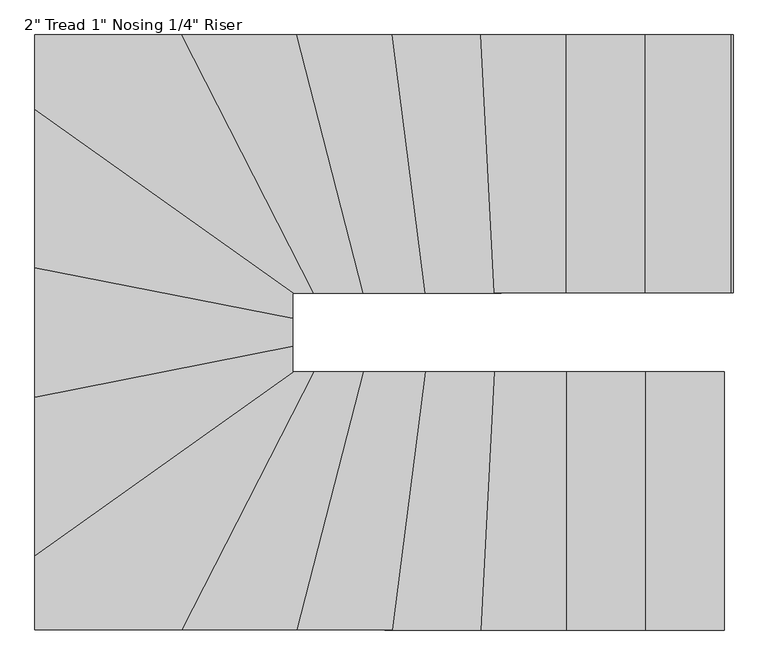
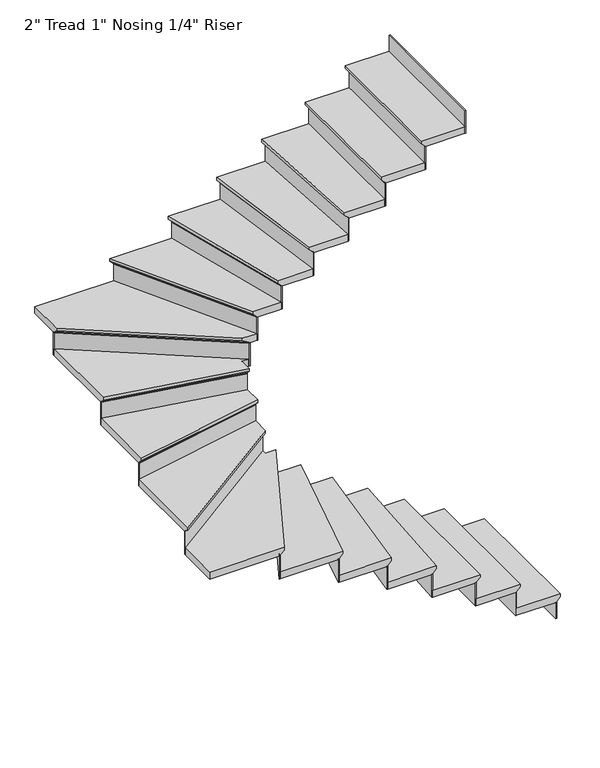
"""IFC4 building model written with IfcOpenShell, lengths in millimetres: stair flight geometry."""

from ifc_helpers import new_model, si_unit, origin, place, context, project, spatial, faceted_brep, source, transform, mapped, element, save


def stair_flight_52655b22(model_context):
    return source(origin(), model_context, "Body", "Brep", [
        faceted_brep([(-13262.6440752, 4370.5418963, 150.2833333), (-13262.6440752, 4370.5418963, 169.3333333), (-13262.6440752, 3456.1418963, 169.3333333), (-13262.6440752, 3456.1418963, 150.2833333), (-13288.0440752, 4370.5418963, 124.8833333), (-13288.0440752, 3456.1418963, 124.8833333), (-13567.4440752, 4370.5418963, 169.3333333), (-13567.4440752, 3456.1418963, 169.3333333), (-13288.0440752, 3456.1418963, 118.5333333), (-13567.4440752, 3456.1418963, 118.5333333), (-13567.4440752, 4370.5418963, 118.5333333), (-13288.0440752, 4370.5418963, 118.5333333)], [[[0, 1, 2, 3]], [[4, 0, 3, 5]], [[2, 1, 6, 7]], [[8, 9, 10, 11]], [[2, 7, 9, 8, 5, 3]], [[8, 11, 4, 5]], [[6, 1, 0, 4, 11, 10]], [[7, 6, 10, 9]]]),
        faceted_brep([(-13288.0440752, 4370.5418963, 118.5333333), (-13288.0440752, 4370.5418963, 0.0), (-13294.3940752, 4370.5418963, 0.0), (-13294.3940752, 4370.5418963, 118.5333333), (-13288.0440752, 3456.1418963, 118.5333333), (-13294.3940752, 3456.1418963, 118.5333333), (-13294.3940752, 3456.1418963, 0.0), (-13288.0440752, 3456.1418963, 0.0)], [[[0, 1, 2, 3]], [[4, 5, 6, 7]], [[1, 0, 4, 7]], [[2, 1, 7, 6]], [[3, 2, 6, 5]], [[0, 3, 5, 4]]]),
        faceted_brep([(-13567.4440752, 4370.5418963, 287.8666667), (-13567.4440752, 4370.5418963, 118.5333333), (-13573.7940752, 4370.5418963, 118.5333333), (-13573.7940752, 4370.5418963, 287.8666667), (-13567.4440752, 3456.1418963, 287.8666667), (-13573.7940752, 3456.1418963, 287.8666667), (-13573.7940752, 3456.1418963, 118.5333333), (-13567.4440752, 3456.1418963, 118.5333333)], [[[0, 1, 2, 3]], [[4, 5, 6, 7]], [[1, 0, 4, 7]], [[2, 1, 7, 6]], [[3, 2, 6, 5]], [[0, 3, 5, 4]]]),
        faceted_brep([(-13542.0440752, 3456.1418963, 338.6666667), (-13542.0440752, 4370.5418963, 338.6666667), (-13846.8440752, 4370.5418963, 338.6666667), (-13846.8440752, 3456.1418963, 338.6666667), (-13567.4440752, 3456.1418963, 287.8666667), (-13846.8440752, 3456.1418963, 287.8666667), (-13846.8440752, 4370.5418963, 287.8666667), (-13567.4440752, 4370.5418963, 287.8666667), (-13567.4440752, 3456.1418963, 294.2166667), (-13542.0440752, 3456.1418963, 319.6166667), (-13567.4440752, 4370.5418963, 294.2166667), (-13542.0440752, 4370.5418963, 319.6166667)], [[[0, 1, 2, 3]], [[4, 5, 6, 7]], [[0, 3, 5, 4, 8, 9]], [[4, 7, 10, 8]], [[2, 1, 11, 10, 7, 6]], [[3, 2, 6, 5]], [[11, 1, 0, 9]], [[10, 11, 9, 8]]]),
        faceted_brep([(-13846.8440752, 4370.5418963, 457.2), (-13846.8440752, 4370.5418963, 287.8666667), (-13853.1940752, 4370.5418963, 287.8666667), (-13853.1940752, 4370.5418963, 457.2), (-13846.8440752, 3456.1418963, 457.2), (-13853.1940752, 3456.1418963, 457.2), (-13853.1940752, 3456.1418963, 287.8666667), (-13846.8440752, 3456.1418963, 287.8666667)], [[[0, 1, 2, 3]], [[4, 5, 6, 7]], [[1, 0, 4, 7]], [[2, 1, 7, 6]], [[3, 2, 6, 5]], [[0, 3, 5, 4]]]),
        faceted_brep([(-13821.4440752, 3456.1418963, 508.0), (-13821.4440752, 4370.5418963, 508.0), (-14102.5112367, 4370.5418963, 508.0), (-14150.0455071, 3456.1418963, 508.0), (-13846.8440752, 3456.1418963, 457.2), (-14150.0455071, 3456.1418963, 457.2), (-14102.5112367, 4370.5418963, 457.2), (-13846.8440752, 4370.5418963, 457.2), (-13846.8440752, 3456.1418963, 463.55), (-13821.4440752, 3456.1418963, 488.95), (-13846.8440752, 4370.5418963, 463.55), (-13821.4440752, 4370.5418963, 488.95)], [[[0, 1, 2, 3]], [[4, 5, 6, 7]], [[0, 3, 5, 4, 8, 9]], [[4, 7, 10, 8]], [[2, 1, 11, 10, 7, 6]], [[3, 2, 6, 5]], [[11, 1, 0, 9]], [[10, 11, 9, 8]]]),
        faceted_brep([(-14102.5112367, 4370.5418963, 626.5333333), (-14102.5112367, 4370.5418963, 457.2), (-14108.8698108, 4370.5418963, 457.2), (-14108.8698108, 4370.5418963, 626.5333333), (-14150.0455071, 3456.1418963, 626.5333333), (-14156.4040812, 3456.1418963, 626.5333333), (-14156.4040812, 3456.1418963, 457.2), (-14150.0455071, 3456.1418963, 457.2)], [[[0, 1, 2, 3]], [[4, 5, 6, 7]], [[1, 0, 4, 7]], [[2, 1, 7, 6]], [[3, 2, 6, 5]], [[0, 3, 5, 4]]]),
        faceted_brep([(-14124.6112104, 3456.1418963, 677.3333333), (-14077.07694, 4370.5418963, 677.3333333), (-14346.6779365, 4370.5418963, 677.3333333), (-14465.0339881, 3456.1418963, 677.3333333), (-14150.0455071, 3456.1418963, 626.5333333), (-14465.0339881, 3456.1418963, 626.5333333), (-14346.6779365, 4370.5418963, 626.5333333), (-14102.5112367, 4370.5418963, 626.5333333), (-14150.0455071, 3456.1418963, 632.8833333), (-14124.6112104, 3456.1418963, 658.2833333), (-14102.5112367, 4370.5418963, 632.8833333), (-14077.07694, 4370.5418963, 658.2833333)], [[[0, 1, 2, 3]], [[4, 5, 6, 7]], [[0, 3, 5, 4, 8, 9]], [[4, 7, 10, 8]], [[2, 1, 11, 10, 7, 6]], [[3, 2, 6, 5]], [[11, 1, 0, 9]], [[10, 11, 9, 8]]]),
        faceted_brep([(-14346.6779365, 4370.5418963, 795.8666667), (-14346.6779365, 4370.5418963, 626.5333333), (-14353.0809083, 4370.5418963, 626.5333333), (-14353.0809083, 4370.5418963, 795.8666667), (-14465.0339881, 3456.1418963, 795.8666667), (-14471.4369599, 3456.1418963, 795.8666667), (-14471.4369599, 3456.1418963, 626.5333333), (-14465.0339881, 3456.1418963, 626.5333333)], [[[0, 1, 2, 3]], [[4, 5, 6, 7]], [[1, 0, 4, 7]], [[2, 1, 7, 6]], [[3, 2, 6, 5]], [[0, 3, 5, 4]]]),
        faceted_brep([(-14439.422101, 3456.1418963, 846.6666667), (-14321.0660494, 4370.5418963, 846.6666667), (-14568.305159, 4370.5418963, 846.6666667), (-14803.4356064, 3456.1418963, 846.6666667), (-14465.0339881, 3456.1418963, 795.8666667), (-14803.4356064, 3456.1418963, 795.8666667), (-14568.305159, 4370.5418963, 795.8666667), (-14346.6779365, 4370.5418963, 795.8666667), (-14465.0339881, 3456.1418963, 802.2166667), (-14439.422101, 3456.1418963, 827.6166667), (-14346.6779365, 4370.5418963, 802.2166667), (-14321.0660494, 4370.5418963, 827.6166667)], [[[0, 1, 2, 3]], [[4, 5, 6, 7]], [[0, 3, 5, 4, 8, 9]], [[4, 7, 10, 8]], [[2, 1, 11, 10, 7, 6]], [[3, 2, 6, 5]], [[11, 1, 0, 9]], [[10, 11, 9, 8]]]),
        faceted_brep([(-14568.305159, 4370.5418963, 965.2), (-14568.305159, 4370.5418963, 795.8666667), (-14574.8617358, 4370.5418963, 795.8666667), (-14574.8617358, 4370.5418963, 965.2), (-14803.4356064, 3456.1418963, 965.2), (-14809.9921832, 3456.1418963, 965.2), (-14809.9921832, 3456.1418963, 795.8666667), (-14803.4356064, 3456.1418963, 795.8666667)], [[[0, 1, 2, 3]], [[4, 5, 6, 7]], [[1, 0, 4, 7]], [[2, 1, 7, 6]], [[3, 2, 6, 5]], [[0, 3, 5, 4]]]),
        faceted_brep([(-14777.2092989, 3456.1418963, 1016.0), (-14542.0788515, 4370.5418963, 1016.0), (-14744.651795, 4370.5418963, 1016.0), (-15213.4764164, 3456.1418963, 1016.0), (-14803.4356064, 3456.1418963, 965.2), (-15213.4764164, 3456.1418963, 965.2), (-14744.651795, 4370.5418963, 965.2), (-14568.305159, 4370.5418963, 965.2), (-14803.4356064, 3456.1418963, 971.55), (-14777.2092989, 3456.1418963, 996.95), (-14568.305159, 4370.5418963, 971.55), (-14542.0788515, 4370.5418963, 996.95)], [[[0, 1, 2, 3]], [[4, 5, 6, 7]], [[0, 3, 5, 4, 8, 9]], [[4, 7, 10, 8]], [[2, 1, 11, 10, 7, 6]], [[3, 2, 6, 5]], [[11, 1, 0, 9]], [[10, 11, 9, 8]]]),
        faceted_brep([(-14744.651795, 4370.5418963, 1134.5333333), (-14744.651795, 4370.5418963, 965.2), (-14751.7877782, 4370.5418963, 965.2), (-14751.7877782, 4370.5418963, 1134.5333333), (-15213.4764164, 3456.1418963, 1134.5333333), (-15220.6123995, 3456.1418963, 1134.5333333), (-15220.6123995, 3456.1418963, 965.2), (-15213.4764164, 3456.1418963, 965.2)], [[[0, 1, 2, 3]], [[4, 5, 6, 7]], [[1, 0, 4, 7]], [[2, 1, 7, 6]], [[3, 2, 6, 5]], [[0, 3, 5, 4]]]),
        faceted_brep([(-15704.7757671, 3749.82303, 1185.3333333), (-15704.7757671, 3456.1418963, 1185.3333333), (-15184.9324838, 3456.1418963, 1185.3333333), (-14716.1078625, 4370.5418963, 1185.3333333), (-14790.3757671, 4370.5418963, 1185.3333333), (-14790.3757671, 4400.0969791, 1185.3333333), (-15704.7757671, 3456.1418963, 1134.5333333), (-15704.7757671, 3749.82303, 1134.5333333), (-14790.3757671, 4400.0969791, 1134.5333333), (-14790.3757671, 4370.5418963, 1134.5333333), (-14744.651795, 4370.5418963, 1134.5333333), (-15213.4764164, 3456.1418963, 1134.5333333), (-15213.4764164, 3456.1418963, 1140.8833333), (-15184.9324838, 3456.1418963, 1166.2833333), (-14744.651795, 4370.5418963, 1140.8833333), (-14716.1078625, 4370.5418963, 1166.2833333)], [[[0, 1, 2, 3, 4, 5]], [[6, 7, 8, 9, 10, 11]], [[1, 0, 7, 6]], [[2, 1, 6, 11, 12, 13]], [[11, 10, 14, 12]], [[4, 3, 15, 14, 10, 9]], [[5, 4, 9, 8]], [[0, 5, 8, 7]], [[15, 3, 2, 13]], [[14, 15, 13, 12]]]),
        faceted_brep([(-14790.3757671, 4400.0969791, 1303.8666667), (-14790.3757671, 4400.0969791, 1134.5333333), (-14790.3757671, 4407.8889539, 1134.5333333), (-14790.3757671, 4407.8889539, 1303.8666667), (-15704.7757671, 3749.82303, 1303.8666667), (-15704.7757671, 3757.6150048, 1303.8666667), (-15704.7757671, 3757.6150048, 1134.5333333), (-15704.7757671, 3749.82303, 1134.5333333)], [[[0, 1, 2, 3]], [[4, 5, 6, 7]], [[1, 0, 4, 7]], [[2, 1, 7, 6]], [[3, 2, 6, 5]], [[0, 3, 5, 4]]]),
        faceted_brep([(-15704.7757671, 3718.6551308, 1354.6666667), (-14790.3757671, 4368.9290799, 1354.6666667), (-14790.3757671, 4486.5510662, 1354.6666667), (-15704.7757671, 4306.3102099, 1354.6666667), (-15704.7757671, 3749.82303, 1303.8666667), (-15704.7757671, 4306.3102099, 1303.8666667), (-14790.3757671, 4486.5510662, 1303.8666667), (-14790.3757671, 4400.0969791, 1303.8666667), (-15704.7757671, 3749.82303, 1310.2166667), (-15704.7757671, 3718.6551308, 1335.6166667), (-14790.3757671, 4400.0969791, 1310.2166667), (-14790.3757671, 4368.9290799, 1335.6166667)], [[[0, 1, 2, 3]], [[4, 5, 6, 7]], [[0, 3, 5, 4, 8, 9]], [[4, 7, 10, 8]], [[2, 1, 11, 10, 7, 6]], [[3, 2, 6, 5]], [[11, 1, 0, 9]], [[10, 11, 9, 8]]]),
        faceted_brep([(-14790.3757671, 4486.5510662, 1473.2), (-14790.3757671, 4486.5510662, 1303.8666667), (-14790.3757671, 4493.0232516, 1303.8666667), (-14790.3757671, 4493.0232516, 1473.2), (-15704.7757671, 4306.3102099, 1473.2), (-15704.7757671, 4312.7823953, 1473.2), (-15704.7757671, 4312.7823953, 1303.8666667), (-15704.7757671, 4306.3102099, 1303.8666667)], [[[0, 1, 2, 3]], [[4, 5, 6, 7]], [[1, 0, 4, 7]], [[2, 1, 7, 6]], [[3, 2, 6, 5]], [[0, 3, 5, 4]]]),
        faceted_brep([(-15704.7757671, 4280.4214681, 1524.0), (-14790.3757671, 4460.6623244, 1524.0), (-14790.3757671, 4585.7102099, 1524.0), (-15704.7757671, 4765.9510662, 1524.0), (-15704.7757671, 4306.3102099, 1473.2), (-15704.7757671, 4765.9510662, 1473.2), (-14790.3757671, 4585.7102099, 1473.2), (-14790.3757671, 4486.5510662, 1473.2), (-15704.7757671, 4306.3102099, 1479.55), (-15704.7757671, 4280.4214681, 1504.95), (-14790.3757671, 4486.5510662, 1479.55), (-14790.3757671, 4460.6623244, 1504.95)], [[[0, 1, 2, 3]], [[4, 5, 6, 7]], [[0, 3, 5, 4, 8, 9]], [[4, 7, 10, 8]], [[2, 1, 11, 10, 7, 6]], [[3, 2, 6, 5]], [[11, 1, 0, 9]], [[10, 11, 9, 8]]]),
        faceted_brep([(-14790.3757671, 4585.7102099, 1642.5333333), (-14790.3757671, 4585.7102099, 1473.2), (-14790.3757671, 4592.1823953, 1473.2), (-14790.3757671, 4592.1823953, 1642.5333333), (-15704.7757671, 4765.9510662, 1642.5333333), (-15704.7757671, 4772.4232516, 1642.5333333), (-15704.7757671, 4772.4232516, 1473.2), (-15704.7757671, 4765.9510662, 1473.2)], [[[0, 1, 2, 3]], [[4, 5, 6, 7]], [[1, 0, 4, 7]], [[2, 1, 7, 6]], [[3, 2, 6, 5]], [[0, 3, 5, 4]]]),
        faceted_brep([(-15704.7757671, 4740.0623244, 1693.3333333), (-14790.3757671, 4559.8214681, 1693.3333333), (-14790.3757671, 4649.9418963, 1693.3333333), (-14744.2802925, 4649.9418963, 1693.3333333), (-15704.7757671, 5332.9965609, 1693.3333333), (-15704.7757671, 4765.9510662, 1642.5333333), (-15704.7757671, 5332.9965609, 1642.5333333), (-14744.2802925, 4649.9418963, 1642.5333333), (-14790.3757671, 4649.9418963, 1642.5333333), (-14790.3757671, 4585.7102099, 1642.5333333), (-15704.7757671, 4765.9510662, 1648.8833333), (-15704.7757671, 4740.0623244, 1674.2833333), (-14790.3757671, 4585.7102099, 1648.8833333), (-14790.3757671, 4559.8214681, 1674.2833333)], [[[0, 1, 2, 3, 4]], [[5, 6, 7, 8, 9]], [[0, 4, 6, 5, 10, 11]], [[5, 9, 12, 10]], [[2, 1, 13, 12, 9, 8]], [[3, 2, 8, 7]], [[4, 3, 7, 6]], [[13, 1, 0, 11]], [[12, 13, 11, 10]]]),
        faceted_brep([(-14744.2802925, 4649.9418963, 1811.8666667), (-14744.2802925, 4649.9418963, 1642.5333333), (-14733.3234, 4649.9418963, 1642.5333333), (-14733.3234, 4649.9418963, 1811.8666667), (-15704.7757671, 5332.9965609, 1811.8666667), (-15704.7757671, 5340.7885357, 1811.8666667), (-15704.7757671, 5340.7885357, 1642.5333333), (-15704.7757671, 5332.9965609, 1642.5333333)], [[[0, 1, 2, 3]], [[4, 5, 6, 7]], [[1, 0, 4, 7]], [[2, 1, 7, 6]], [[3, 2, 6, 5]], [[0, 3, 5, 4]]]),
        faceted_brep([(-15156.3885513, 5564.3418963, 1862.6666667), (-15704.7757671, 5564.3418963, 1862.6666667), (-15704.7757671, 5301.8286618, 1862.6666667), (-14788.1078625, 4649.9418963, 1862.6666667), (-14687.56393, 4649.9418963, 1862.6666667), (-15704.7757671, 5564.3418963, 1811.8666667), (-15156.3885513, 5564.3418963, 1811.8666667), (-14687.56393, 4649.9418963, 1811.8666667), (-14744.2802925, 4649.9418963, 1811.8666667), (-15704.7757671, 5332.9965609, 1811.8666667), (-15704.7757671, 5332.9965609, 1818.2166667), (-15704.7757671, 5301.8286618, 1843.6166667), (-14744.2802925, 4649.9418963, 1818.2166667), (-14788.1078625, 4649.9418963, 1843.6166667)], [[[0, 1, 2, 3, 4]], [[5, 6, 7, 8, 9]], [[1, 0, 6, 5]], [[2, 1, 5, 9, 10, 11]], [[9, 8, 12, 10]], [[4, 3, 13, 12, 8, 7]], [[0, 4, 7, 6]], [[13, 3, 2, 11]], [[12, 13, 11, 10]]]),
        faceted_brep([(-14687.56393, 4649.9418963, 1981.2), (-14687.56393, 4649.9418963, 1811.8666667), (-14680.4279468, 4649.9418963, 1811.8666667), (-14680.4279468, 4649.9418963, 1981.2), (-15156.3885513, 5564.3418963, 1981.2), (-15149.2525682, 5564.3418963, 1981.2), (-15149.2525682, 5564.3418963, 1811.8666667), (-15156.3885513, 5564.3418963, 1811.8666667)], [[[0, 1, 2, 3]], [[4, 5, 6, 7]], [[1, 0, 4, 7]], [[2, 1, 7, 6]], [[3, 2, 6, 5]], [[0, 3, 5, 4]]]),
        faceted_brep([(-15184.9324838, 5564.3418963, 2032.0), (-14716.1078625, 4649.9418963, 2032.0), (-14515.852544, 4649.9418963, 2032.0), (-14750.9829914, 5564.3418963, 2032.0), (-15156.3885513, 5564.3418963, 1981.2), (-14750.9829914, 5564.3418963, 1981.2), (-14515.852544, 4649.9418963, 1981.2), (-14687.56393, 4649.9418963, 1981.2), (-15156.3885513, 5564.3418963, 1987.55), (-15184.9324838, 5564.3418963, 2012.95), (-14687.56393, 4649.9418963, 1987.55), (-14716.1078625, 4649.9418963, 2012.95)], [[[0, 1, 2, 3]], [[4, 5, 6, 7]], [[0, 3, 5, 4, 8, 9]], [[4, 7, 10, 8]], [[2, 1, 11, 10, 7, 6]], [[3, 2, 6, 5]], [[11, 1, 0, 9]], [[10, 11, 9, 8]]]),
        faceted_brep([(-14515.852544, 4649.9418963, 2150.5333333), (-14515.852544, 4649.9418963, 1981.2), (-14509.2959672, 4649.9418963, 1981.2), (-14509.2959672, 4649.9418963, 2150.5333333), (-14750.9829914, 5564.3418963, 2150.5333333), (-14744.4264146, 5564.3418963, 2150.5333333), (-14744.4264146, 5564.3418963, 1981.2), (-14750.9829914, 5564.3418963, 1981.2)], [[[0, 1, 2, 3]], [[4, 5, 6, 7]], [[1, 0, 4, 7]], [[2, 1, 7, 6]], [[3, 2, 6, 5]], [[0, 3, 5, 4]]]),
        faceted_brep([(-14777.2092989, 5564.3418963, 2201.3333333), (-14542.0788515, 4649.9418963, 2201.3333333), (-14295.4541623, 4649.9418963, 2201.3333333), (-14413.8102139, 5564.3418963, 2201.3333333), (-14750.9829914, 5564.3418963, 2150.5333333), (-14413.8102139, 5564.3418963, 2150.5333333), (-14295.4541623, 4649.9418963, 2150.5333333), (-14515.852544, 4649.9418963, 2150.5333333), (-14750.9829914, 5564.3418963, 2156.8833333), (-14777.2092989, 5564.3418963, 2182.2833333), (-14515.852544, 4649.9418963, 2156.8833333), (-14542.0788515, 4649.9418963, 2182.2833333)], [[[0, 1, 2, 3]], [[4, 5, 6, 7]], [[0, 3, 5, 4, 8, 9]], [[4, 7, 10, 8]], [[2, 1, 11, 10, 7, 6]], [[3, 2, 6, 5]], [[11, 1, 0, 9]], [[10, 11, 9, 8]]]),
        faceted_brep([(-14295.4541623, 4649.9418963, 2319.8666667), (-14295.4541623, 4649.9418963, 2150.5333333), (-14289.0511905, 4649.9418963, 2150.5333333), (-14289.0511905, 4649.9418963, 2319.8666667), (-14413.8102139, 5564.3418963, 2319.8666667), (-14407.4072421, 5564.3418963, 2319.8666667), (-14407.4072421, 5564.3418963, 2150.5333333), (-14413.8102139, 5564.3418963, 2150.5333333)], [[[0, 1, 2, 3]], [[4, 5, 6, 7]], [[1, 0, 4, 7]], [[2, 1, 7, 6]], [[3, 2, 6, 5]], [[0, 3, 5, 4]]]),
        faceted_brep([(-14439.422101, 5564.3418963, 2370.6666667), (-14321.0660494, 4649.9418963, 2370.6666667), (-14051.6426433, 4649.9418963, 2370.6666667), (-14099.1769137, 5564.3418963, 2370.6666667), (-14413.8102139, 5564.3418963, 2319.8666667), (-14099.1769137, 5564.3418963, 2319.8666667), (-14051.6426433, 4649.9418963, 2319.8666667), (-14295.4541623, 4649.9418963, 2319.8666667), (-14413.8102139, 5564.3418963, 2326.2166667), (-14439.422101, 5564.3418963, 2351.6166667), (-14295.4541623, 4649.9418963, 2326.2166667), (-14321.0660494, 4649.9418963, 2351.6166667)], [[[0, 1, 2, 3]], [[4, 5, 6, 7]], [[0, 3, 5, 4, 8, 9]], [[4, 7, 10, 8]], [[2, 1, 11, 10, 7, 6]], [[3, 2, 6, 5]], [[11, 1, 0, 9]], [[10, 11, 9, 8]]]),
        faceted_brep([(-14051.6426433, 4649.9418963, 2489.2), (-14051.6426433, 4649.9418963, 2319.8666667), (-14045.2840692, 4649.9418963, 2319.8666667), (-14045.2840692, 4649.9418963, 2489.2), (-14099.1769137, 5564.3418963, 2489.2), (-14092.8183396, 5564.3418963, 2489.2), (-14092.8183396, 5564.3418963, 2319.8666667), (-14099.1769137, 5564.3418963, 2319.8666667)], [[[0, 1, 2, 3]], [[4, 5, 6, 7]], [[1, 0, 4, 7]], [[2, 1, 7, 6]], [[3, 2, 6, 5]], [[0, 3, 5, 4]]]),
        faceted_brep([(-14124.6112104, 5564.3418963, 2540.0), (-14077.07694, 4649.9418963, 2540.0), (-13796.0440752, 4649.9418963, 2540.0), (-13796.0440752, 5564.3418963, 2540.0), (-14099.1769137, 5564.3418963, 2489.2), (-13796.0440752, 5564.3418963, 2489.2), (-13796.0440752, 4649.9418963, 2489.2), (-14051.6426433, 4649.9418963, 2489.2), (-14099.1769137, 5564.3418963, 2495.55), (-14124.6112104, 5564.3418963, 2520.95), (-14051.6426433, 4649.9418963, 2495.55), (-14077.07694, 4649.9418963, 2520.95)], [[[0, 1, 2, 3]], [[4, 5, 6, 7]], [[0, 3, 5, 4, 8, 9]], [[4, 7, 10, 8]], [[2, 1, 11, 10, 7, 6]], [[3, 2, 6, 5]], [[11, 1, 0, 9]], [[10, 11, 9, 8]]]),
        faceted_brep([(-13796.0440752, 4649.9418963, 2658.5333333), (-13796.0440752, 4649.9418963, 2489.2), (-13789.6940752, 4649.9418963, 2489.2), (-13789.6940752, 4649.9418963, 2658.5333333), (-13796.0440752, 5564.3418963, 2658.5333333), (-13789.6940752, 5564.3418963, 2658.5333333), (-13789.6940752, 5564.3418963, 2489.2), (-13796.0440752, 5564.3418963, 2489.2)], [[[0, 1, 2, 3]], [[4, 5, 6, 7]], [[1, 0, 4, 7]], [[2, 1, 7, 6]], [[3, 2, 6, 5]], [[0, 3, 5, 4]]]),
        faceted_brep([(-13821.4440752, 5564.3418963, 2709.3333333), (-13821.4440752, 4649.9418963, 2709.3333333), (-13516.6440752, 4649.9418963, 2709.3333333), (-13516.6440752, 5564.3418963, 2709.3333333), (-13796.0440752, 5564.3418963, 2658.5333333), (-13516.6440752, 5564.3418963, 2658.5333333), (-13516.6440752, 4649.9418963, 2658.5333333), (-13796.0440752, 4649.9418963, 2658.5333333), (-13796.0440752, 5564.3418963, 2664.8833333), (-13821.4440752, 5564.3418963, 2690.2833333), (-13796.0440752, 4649.9418963, 2664.8833333), (-13821.4440752, 4649.9418963, 2690.2833333)], [[[0, 1, 2, 3]], [[4, 5, 6, 7]], [[0, 3, 5, 4, 8, 9]], [[4, 7, 10, 8]], [[2, 1, 11, 10, 7, 6]], [[3, 2, 6, 5]], [[11, 1, 0, 9]], [[10, 11, 9, 8]]]),
        faceted_brep([(-13516.6440752, 4649.9418963, 2827.8666667), (-13516.6440752, 4649.9418963, 2658.5333333), (-13510.2940752, 4649.9418963, 2658.5333333), (-13510.2940752, 4649.9418963, 2827.8666667), (-13516.6440752, 5564.3418963, 2827.8666667), (-13510.2940752, 5564.3418963, 2827.8666667), (-13510.2940752, 5564.3418963, 2658.5333333), (-13516.6440752, 5564.3418963, 2658.5333333)], [[[0, 1, 2, 3]], [[4, 5, 6, 7]], [[1, 0, 4, 7]], [[2, 1, 7, 6]], [[3, 2, 6, 5]], [[0, 3, 5, 4]]]),
        faceted_brep([(-13237.2440752, 4649.9418963, 2997.2), (-13237.2440752, 4649.9418963, 2827.8666667), (-13230.8940752, 4649.9418963, 2827.8666667), (-13230.8940752, 4649.9418963, 2997.2), (-13237.2440752, 5564.3418963, 2997.2), (-13230.8940752, 5564.3418963, 2997.2), (-13230.8940752, 5564.3418963, 2827.8666667), (-13237.2440752, 5564.3418963, 2827.8666667)], [[[0, 1, 2, 3]], [[4, 5, 6, 7]], [[1, 0, 4, 7]], [[2, 1, 7, 6]], [[3, 2, 6, 5]], [[0, 3, 5, 4]]]),
        faceted_brep([(-13542.0440752, 5564.3418963, 2878.6666667), (-13542.0440752, 4649.9418963, 2878.6666667), (-13237.2440752, 4649.9418963, 2878.6666667), (-13237.2440752, 5564.3418963, 2878.6666667), (-13516.6440752, 5564.3418963, 2827.8666667), (-13237.2440752, 5564.3418963, 2827.8666667), (-13237.2440752, 4649.9418963, 2827.8666667), (-13516.6440752, 4649.9418963, 2827.8666667), (-13516.6440752, 5564.3418963, 2834.2166667), (-13542.0440752, 5564.3418963, 2859.6166667), (-13516.6440752, 4649.9418963, 2834.2166667), (-13542.0440752, 4649.9418963, 2859.6166667)], [[[0, 1, 2, 3]], [[4, 5, 6, 7]], [[0, 3, 5, 4, 8, 9]], [[4, 7, 10, 8]], [[2, 1, 11, 10, 7, 6]], [[3, 2, 6, 5]], [[11, 1, 0, 9]], [[10, 11, 9, 8]]]),
    ])


if __name__ == "__main__":
    model = new_model("IFC4")
    model_context = context("Model", 3, world=origin())
    ifc_project = project(units=[si_unit("LENGTHUNIT", "METRE", prefix="MILLI")], contexts=[model_context])
    site = spatial("IfcSite", under=ifc_project)
    building = spatial("IfcBuilding", under=site)
    placement = place(None, origin())
    stair_flight_shape = stair_flight_52655b22(model_context)
    element("IfcStairFlight", 1, ObjectType="2\" Tread 1\" Nosing 1/4\" Riser", at=placement, inside=building, context=model_context, shape_type="MappedRepresentation", body=[
        mapped(stair_flight_shape, transform((0.0, 0.0, 0.0), x_axis=(1.0, 0.0, 0.0), y_axis=(0.0, 1.0, 0.0), z_axis=(0.0, 0.0, 1.0))),
    ])
    save(model, "model.ifc")
